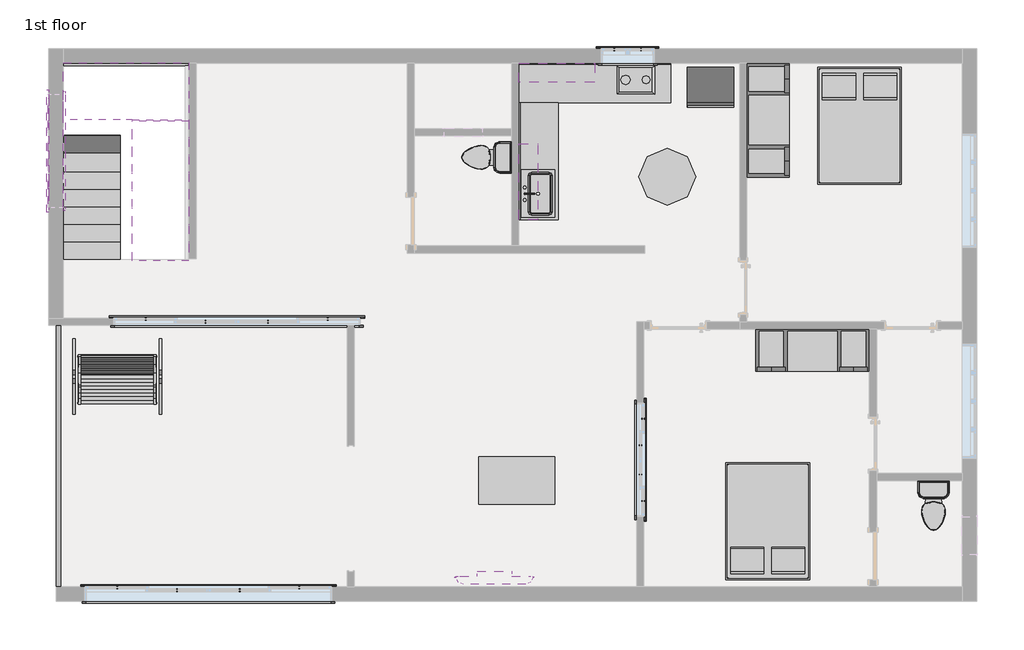
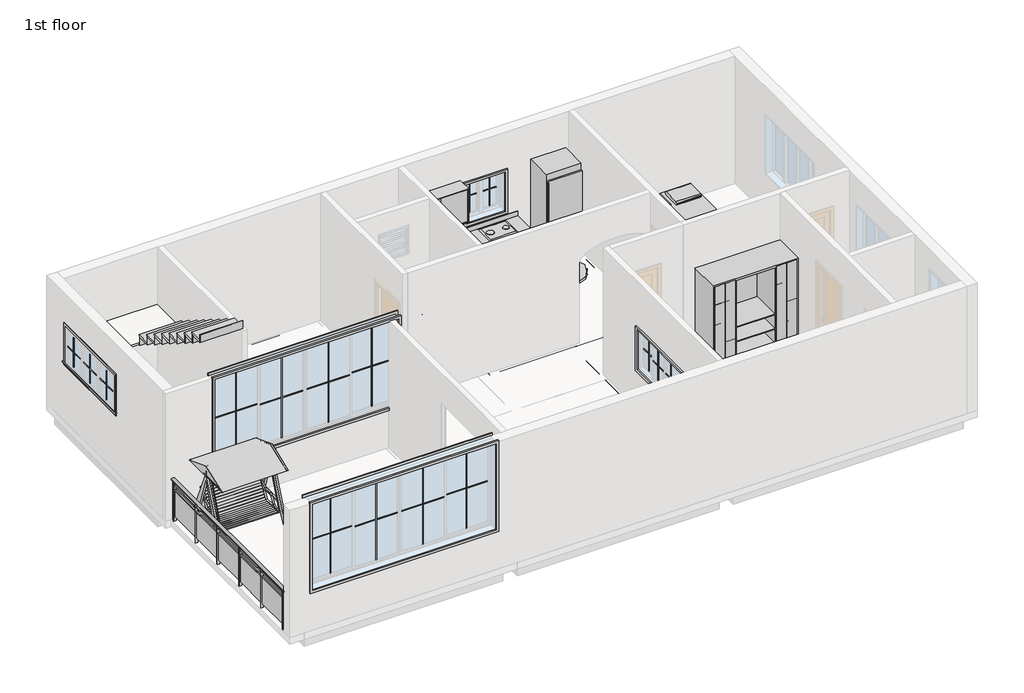
# One storey, part 2 of 2: 30 proxies, 16 furniture elements, 8 beams, 3 flow terminals, 2 stair flights, 1 railing, 1 slab.
"""IFC4 building model written with IfcOpenShell, lengths in millimetres."""

from ifc_helpers import new_model, si_unit, point, frame, origin, place, context, project, spatial, polyline, ellipse_curve, trimmed, outline, extrude, faceted_brep, transform, mapped, element, save
from ifc_brep_helpers import plane_surface, extruded_surface, advanced_brep
from components import proxy_3c1fa1d0, proxy_caef4acf, muntin_pattern_2x2_muntin_pattern_2x2_31a16349, muntin_pattern_2x2_muntin_pattern_2x2_a56fcb99, muntin_pattern_2x2_muntin_pattern_2x2_c58f38d7, muntin_pattern_2x2_muntin_pattern_2x2_b3fe6957, muntin_pattern_2x2_muntin_pattern_2x2_3e0ecaf2, muntin_pattern_2x2_muntin_pattern_2x2_51cb8927, proxy_19935bb1, trim_window_exterior_flat_with_sill_3c945769, trim_window_exterior_flat_with_sill_7b949e88, trim_window_exterior_flat_with_sill_41619996, trim_window_exterior_flat_with_sill_170b7f0e, trim_window_interior_flat_picture_frame_0edfbaa2, trim_window_interior_flat_picture_frame_687edbe0, trim_window_interior_flat_picture_frame_51c85655, trim_window_interior_flat_picture_frame_cc79b2fe, flow_terminal_4d548711, toilet_domestic_3d_toilet_domestic_3d_ba6479b0, toilet_domestic_3d_toilet_domestic_3d_30431060, furniture_0762_x_0762mm_a8fad5e2, furniture_f87f75a4, furniture_97fe820d, furniture_b58f7881, furniture_deb1c5d1, furniture_078eb3f3, furniture_88072bd9, furniture_0b81fedb, furniture_acc2807d, furniture_52f35bf4, furniture_f491f192, non_monolithic_landing_e0ece5e3, stair_flight_342035e6, stair_flight_9be7654d

model = new_model("IFC4")

# Units and contexts
model_context = context("Model", 3, world=origin())
ifc_project = project(units=[si_unit("LENGTHUNIT", "METRE", prefix="MILLI")], contexts=[model_context])

# Site, building, storey
site = spatial("IfcSite", under=ifc_project)
building = spatial("IfcBuilding", under=site)
storey = spatial("IfcBuildingStorey", under=building, Name="1st floor", Elevation=3810.0)

# Beams
placement = place(None, origin())
element("IfcBeam", 1, ObjectType="Concrete-Rectangular Beam", at=placement, inside=storey, context=model_context, shape_type="Brep", body=[
    faceted_brep([(-12643.368339, 9510.993496, 3810.0), (-12643.368339, 9282.393496, 3810.0), (-10681.218339, 9282.393496, 3810.0), (-10452.618339, 9282.393496, 3810.0), (-7176.018339, 9282.393496, 3810.0), (-6947.418339, 9282.393496, 3810.0), (-5499.618339, 9282.393496, 3810.0), (-5271.018339, 9282.393496, 3810.0), (-3492.916739, 9282.393496, 3810.0), (-3264.316739, 9282.393496, 3810.0), (-1842.018339, 9282.393496, 3810.0), (-1613.418339, 9282.393496, 3810.0), (1790.181661, 9282.393496, 3810.0), (1790.181661, 9510.993496, 3810.0), (-1575.318339, 9510.993496, 3810.0), (-1575.318339, 9320.493496, 3810.0), (-1880.118339, 9320.493496, 3810.0), (-1880.118339, 9510.993496, 3810.0), (-6909.318339, 9510.993496, 3810.0), (-6909.318339, 9320.493496, 3810.0), (-7214.118339, 9320.493496, 3810.0), (-7214.118339, 9510.993496, 3810.0), (-10414.518339, 9510.993496, 3810.0), (-10414.518339, 9320.493496, 3810.0), (-10719.318339, 9320.493496, 3810.0), (-10719.318339, 9510.993496, 3810.0), (-12643.368339, 9282.393496, 3505.2), (-10681.218339, 9282.393496, 3505.2), (-10452.618339, 9282.393496, 3505.2), (-7176.018339, 9282.393496, 3505.2), (-6947.418339, 9282.393496, 3505.2), (-5499.618339, 9282.393496, 3505.2), (-5271.018339, 9282.393496, 3505.2), (-3492.916739, 9282.393496, 3505.2), (-3264.316739, 9282.393496, 3505.2), (-1842.018339, 9282.393496, 3505.2), (-1613.418339, 9282.393496, 3505.2), (1790.181661, 9282.393496, 3505.2), (-12643.368339, 9510.993496, 3505.2), (-10719.318339, 9510.993496, 3505.2), (-10719.318339, 9320.493496, 3505.2), (-10414.518339, 9320.493496, 3505.2), (-10414.518339, 9510.993496, 3505.2), (-7214.118339, 9510.993496, 3505.2), (-7214.118339, 9320.493496, 3505.2), (-6909.318339, 9320.493496, 3505.2), (-6909.318339, 9510.993496, 3505.2), (-1880.118339, 9510.993496, 3505.2), (-1880.118339, 9320.493496, 3505.2), (-1575.318339, 9320.493496, 3505.2), (-1575.318339, 9510.993496, 3505.2), (1790.181661, 9510.993496, 3505.2)], [[[0, 1, 2, 3, 4, 5, 6, 7, 8, 9, 10, 11, 12, 13, 14, 15, 16, 17, 18, 19, 20, 21, 22, 23, 24, 25]], [[1, 26, 27, 28, 29, 30, 31, 32, 33, 34, 35, 36, 37, 12, 11, 10, 9, 8, 7, 6, 5, 4, 3, 2]], [[26, 38, 39, 40, 41, 42, 43, 44, 45, 46, 47, 48, 49, 50, 51, 37, 36, 35, 34, 33, 32, 31, 30, 29, 28, 27]], [[13, 51, 50, 14]], [[1, 0, 38, 26]], [[13, 12, 37, 51]], [[41, 23, 22, 42]], [[23, 41, 40, 24]], [[24, 40, 39, 25]], [[38, 0, 25, 39]], [[45, 19, 18, 46]], [[19, 45, 44, 20]], [[20, 44, 43, 21]], [[42, 22, 21, 43]], [[49, 15, 14, 50]], [[15, 49, 48, 16]], [[16, 48, 47, 17]], [[46, 18, 17, 47]]]),
])
element("IfcBeam", 2, ObjectType="Concrete-Rectangular Beam", at=placement, inside=storey, context=model_context, shape_type="Brep", body=[
    faceted_brep([(1790.181661, 913.093496, 3810.0), (2018.781661, 913.093496, 3810.0), (2018.781661, 4958.043496, 3810.0), (1790.181661, 4958.043496, 3810.0), (1790.181661, 2792.693496, 3810.0), (1790.181661, 2564.093496, 3810.0), (1790.181661, 913.093496, 3505.2), (1790.181661, 4958.043496, 3505.2), (1790.181661, 2792.693496, 3505.2), (1790.181661, 2564.093496, 3505.2), (2018.781661, 913.093496, 3505.2), (2018.781661, 4958.043496, 3505.2)], [[[0, 1, 2, 3, 4, 5]], [[6, 0, 5, 4, 3, 7, 8, 9]], [[10, 6, 9, 8, 7, 11]], [[1, 10, 11, 2]], [[1, 0, 6, 10]], [[3, 2, 11, 7]]]),
    faceted_brep([(1790.181661, 9244.293496, 3810.0), (2018.781661, 9244.293496, 3810.0), (2018.781661, 9244.293496, 3505.2), (1790.181661, 9244.293496, 3505.2), (2018.781661, 5262.843496, 3810.0), (1790.181661, 5262.843496, 3810.0), (1790.181661, 5262.843496, 3505.2), (2018.781661, 5262.843496, 3505.2), (1790.181661, 6443.943496, 3810.0), (1790.181661, 6215.343496, 3810.0), (1790.181661, 6443.943496, 3505.2), (1790.181661, 6215.343496, 3505.2)], [[[0, 1, 2, 3]], [[4, 5, 6, 7]], [[1, 0, 8, 9, 5, 4]], [[0, 3, 10, 11, 6, 5, 9, 8]], [[3, 2, 7, 6, 11, 10]], [[2, 1, 4, 7]]]),
])
element("IfcBeam", 3, ObjectType="Concrete-Rectangular Beam", at=placement, inside=storey, context=model_context, shape_type="SweptSolid", body=[
    extrude(outline(polyline([(-6947.418339, 8094.943496), (-6947.418339, 8323.543496), (-5499.618339, 8323.543496), (-5499.618339, 8094.943496), (-6947.418339, 8094.943496)])), frame((0.0, 0.0, 3505.2), z_axis=(0.0, 0.0, 1.0), x_axis=(1.0, 0.0, 0.0)), (0.0, 0.0, 1.0), 304.8),
])
element("IfcBeam", 4, ObjectType="Concrete-Rectangular Beam", at=placement, inside=storey, context=model_context, shape_type="Brep", body=[
    faceted_brep([(-6947.418339, 6443.943496, 3810.0), (-6947.418339, 6215.343496, 3810.0), (-5499.618339, 6215.343496, 3810.0), (-5499.618339, 6443.943496, 3810.0), (-6947.418339, 6215.343496, 3505.2), (-5499.618339, 6215.343496, 3505.2), (-6947.418339, 6443.943496, 3505.2), (-5499.618339, 6443.943496, 3505.2)], [[[0, 1, 2, 3]], [[1, 4, 5, 2]], [[4, 6, 7, 5]], [[6, 0, 3, 7]], [[1, 0, 6, 4]], [[3, 2, 5, 7]]]),
    faceted_brep([(1790.181661, 6443.943496, 3810.0), (1790.181661, 6215.343496, 3810.0), (1790.181661, 6215.343496, 3505.2), (1790.181661, 6443.943496, 3505.2), (-5271.018339, 6215.343496, 3810.0), (-5271.018339, 6443.943496, 3810.0), (-5271.018339, 6443.943496, 3505.2), (-5271.018339, 6215.343496, 3505.2), (-1613.418339, 6443.943496, 3810.0), (-1842.018339, 6443.943496, 3810.0), (-3264.316739, 6443.943496, 3810.0), (-3492.916739, 6443.943496, 3810.0), (-3492.916739, 6215.343496, 3810.0), (-3264.316739, 6215.343496, 3810.0), (-1842.018339, 6215.343496, 3810.0), (-1613.418339, 6215.343496, 3810.0), (-3492.916739, 6215.343496, 3505.2), (-3264.316739, 6215.343496, 3505.2), (-1842.018339, 6215.343496, 3505.2), (-1613.418339, 6215.343496, 3505.2), (-3492.916739, 6443.943496, 3505.2), (-3264.316739, 6443.943496, 3505.2), (-1842.018339, 6443.943496, 3505.2), (-1613.418339, 6443.943496, 3505.2)], [[[0, 1, 2, 3]], [[4, 5, 6, 7]], [[1, 0, 8, 9, 10, 11, 5, 4, 12, 13, 14, 15]], [[2, 1, 15, 14, 13, 12, 4, 7, 16, 17, 18, 19]], [[3, 2, 19, 18, 17, 16, 7, 6, 20, 21, 22, 23]], [[0, 3, 23, 22, 21, 20, 6, 5, 11, 10, 9, 8]]]),
])
element("IfcBeam", 5, ObjectType="Concrete-Rectangular Beam", at=placement, inside=storey, context=model_context, shape_type="Brep", body=[
    faceted_brep([(-1842.018339, 913.093496, 3810.0), (-1613.418339, 913.093496, 3810.0), (-1613.418339, 4996.143496, 3810.0), (-1613.418339, 5224.743496, 3810.0), (-1613.418339, 6215.343496, 3810.0), (-1842.018339, 6215.343496, 3810.0), (-1842.018339, 5281.893496, 3810.0), (-1784.868339, 5281.893496, 3810.0), (-1784.868339, 5053.293496, 3810.0), (-1842.018339, 5053.293496, 3810.0), (-1842.018339, 4996.143496, 3810.0), (-1842.018339, 913.093496, 3505.2), (-1842.018339, 5053.293496, 3505.2), (-1842.018339, 4996.143496, 3505.2), (-1613.418339, 913.093496, 3505.2), (-1784.868339, 5053.293496, 3505.2), (-1784.868339, 5281.893496, 3505.2), (-1842.018339, 5281.893496, 3505.2), (-1842.018339, 6215.343496, 3505.2), (-1613.418339, 6215.343496, 3505.2), (-1613.418339, 5224.743496, 3505.2), (-1613.418339, 4996.143496, 3505.2)], [[[0, 1, 2, 3, 4, 5, 6, 7, 8, 9, 10]], [[11, 0, 10, 9, 12, 13]], [[14, 11, 13, 12, 15, 16, 17, 18, 19, 20, 21]], [[1, 14, 21, 20, 19, 4, 3, 2]], [[1, 0, 11, 14]], [[5, 4, 19, 18]], [[8, 15, 12, 9]], [[16, 7, 6, 17]], [[7, 16, 15, 8]], [[5, 18, 17, 6]]]),
    faceted_brep([(-1842.018339, 9282.393496, 3810.0), (-1613.418339, 9282.393496, 3810.0), (-1613.418339, 9282.393496, 3505.2), (-1842.018339, 9282.393496, 3505.2), (-1613.418339, 6443.943496, 3810.0), (-1842.018339, 6443.943496, 3810.0), (-1842.018339, 6443.943496, 3505.2), (-1613.418339, 6443.943496, 3505.2)], [[[0, 1, 2, 3]], [[4, 5, 6, 7]], [[1, 0, 5, 4]], [[3, 2, 7, 6]], [[2, 1, 4, 7]], [[0, 3, 6, 5]]]),
])
element("IfcBeam", 6, ObjectType="Concrete-Rectangular Beam", at=placement, inside=storey, context=model_context, shape_type="SweptSolid", body=[
    extrude(outline(polyline([(-3492.916739, 9282.393496), (-3264.316739, 9282.393496), (-3264.316739, 6443.943496), (-3492.916739, 6443.943496), (-3492.916739, 9282.393496)])), frame((0.0, 0.0, 3505.2), z_axis=(0.0, 0.0, 1.0), x_axis=(1.0, 0.0, 0.0)), (0.0, 0.0, 1.0), 304.8),
    extrude(outline(polyline([(-3492.916739, 6215.343496), (-3264.316739, 6215.343496), (-3264.316739, 5224.743496), (-3492.916739, 5224.743496), (-3492.916739, 6215.343496)])), frame((0.0, 0.0, 3505.2), z_axis=(0.0, 0.0, 1.0), x_axis=(1.0, 0.0, 0.0)), (0.0, 0.0, 1.0), 304.8),
    extrude(outline(polyline([(-3492.916739, 4996.143496), (-3264.316739, 4996.143496), (-3264.316739, 913.093496), (-3492.916739, 913.093496), (-3492.916739, 4996.143496)])), frame((0.0, 0.0, 3505.2), z_axis=(0.0, 0.0, 1.0), x_axis=(1.0, 0.0, 0.0)), (0.0, 0.0, 1.0), 304.8),
])
element("IfcBeam", 7, ObjectType="Concrete-Rectangular Beam", at=placement, inside=storey, context=model_context, shape_type="Brep", body=[
    faceted_brep([(240.781661, 913.093496, 3810.0), (469.381661, 913.093496, 3810.0), (469.381661, 2564.093496, 3810.0), (469.381661, 2792.693496, 3810.0), (469.381661, 4996.143496, 3810.0), (240.781661, 4996.143496, 3810.0), (469.381661, 913.093496, 3505.2), (469.381661, 2564.093496, 3505.2), (469.381661, 2792.693496, 3505.2), (469.381661, 4996.143496, 3505.2), (240.781661, 913.093496, 3505.2), (240.781661, 4996.143496, 3505.2)], [[[0, 1, 2, 3, 4, 5]], [[1, 6, 7, 8, 9, 4, 3, 2]], [[6, 10, 11, 9, 8, 7]], [[10, 0, 5, 11]], [[1, 0, 10, 6]], [[5, 4, 9, 11]]]),
])
element("IfcBeam", 8, ObjectType="Concrete-Rectangular Beam", at=placement, inside=storey, context=model_context, shape_type="SweptSolid", body=[
    extrude(outline(polyline([(1790.181661, 2792.693496), (1790.181661, 2564.093496), (469.381661, 2564.093496), (469.381661, 2792.693496), (1790.181661, 2792.693496)])), frame((0.0, 0.0, 3505.2), z_axis=(0.0, 0.0, 1.0), x_axis=(1.0, 0.0, 0.0)), (0.0, 0.0, 1.0), 304.8),
])

# Proxies
proxy_shape = proxy_3c1fa1d0(model_context)
element("IfcBuildingElementProxy", 9, Name="Cook Top-2 Unit : 12\" x 18\"", ObjectType="Cook Top-2 Unit : 12\" x 18\"", at=placement, inside=storey, context=model_context, shape_type="MappedRepresentation", body=[
    mapped(proxy_shape, transform((-3421.5185434, 8977.593496, 3810.0), x_axis=(0.0, 1.0, 0.0), y_axis=(-1.0, 0.0, 0.0), z_axis=(0.0, 0.0, 1.0))),
])
proxy_2_shape = proxy_caef4acf(model_context)
element("IfcBuildingElementProxy", 10, Name="Cook Top-2 Unit : 16\" x 22\"", ObjectType="Cook Top-2 Unit : 16\" x 22\"", at=placement, inside=storey, context=model_context, shape_type="MappedRepresentation", body=[
    mapped(proxy_2_shape, transform((-3370.7185434, 8977.593496, 3810.0), x_axis=(0.0, 1.0, 0.0), y_axis=(-1.0, 0.0, 0.0), z_axis=(0.0, 0.0, 1.0))),
])
muntin_pattern_2x2_muntin_pattern_2x2_shape = muntin_pattern_2x2_muntin_pattern_2x2_31a16349(model_context)
element("IfcBuildingElementProxy", 11, Name="Muntin Pattern_2x2 : Muntin Pattern_2x2", ObjectType="Muntin Pattern_2x2 : Muntin Pattern_2x2", at=placement, inside=storey, context=model_context, shape_type="MappedRepresentation", body=[
    mapped(muntin_pattern_2x2_muntin_pattern_2x2_shape, transform((-3330.991739, 3615.018496, 4806.95), x_axis=(0.0, -1.0, 0.0), y_axis=(1.0, 0.0, 0.0), z_axis=(0.0, 0.0, 1.0))),
])
element("IfcBuildingElementProxy", 12, Name="Muntin Pattern_2x2 : Muntin Pattern_2x2", ObjectType="Muntin Pattern_2x2 : Muntin Pattern_2x2", at=placement, inside=storey, context=model_context, shape_type="MappedRepresentation", body=[
    mapped(muntin_pattern_2x2_muntin_pattern_2x2_shape, transform((-3375.441739, 3189.568496, 4806.95), x_axis=(0.0, -1.0, 0.0), y_axis=(1.0, 0.0, 0.0), z_axis=(0.0, 0.0, 1.0))),
])
element("IfcBuildingElementProxy", 13, Name="Muntin Pattern_2x2 : Muntin Pattern_2x2", ObjectType="Muntin Pattern_2x2 : Muntin Pattern_2x2", at=placement, inside=storey, context=model_context, shape_type="MappedRepresentation", body=[
    mapped(muntin_pattern_2x2_muntin_pattern_2x2_shape, transform((-3375.441739, 2719.668496, 4806.95), x_axis=(0.0, -1.0, 0.0), y_axis=(1.0, 0.0, 0.0), z_axis=(0.0, 0.0, 1.0))),
])
element("IfcBuildingElementProxy", 14, Name="Muntin Pattern_2x2 : Muntin Pattern_2x2", ObjectType="Muntin Pattern_2x2 : Muntin Pattern_2x2", at=placement, inside=storey, context=model_context, shape_type="MappedRepresentation", body=[
    mapped(muntin_pattern_2x2_muntin_pattern_2x2_shape, transform((-3330.991739, 2294.218496, 4806.95), x_axis=(0.0, -1.0, 0.0), y_axis=(1.0, 0.0, 0.0), z_axis=(0.0, 0.0, 1.0))),
])
muntin_pattern_2x2_muntin_pattern_2x2_2_shape = muntin_pattern_2x2_muntin_pattern_2x2_a56fcb99(model_context)
element("IfcBuildingElementProxy", 15, Name="Muntin Pattern_2x2 : Muntin Pattern_2x2", ObjectType="Muntin Pattern_2x2 : Muntin Pattern_2x2", at=placement, inside=storey, context=model_context, shape_type="MappedRepresentation", body=[
    mapped(muntin_pattern_2x2_muntin_pattern_2x2_2_shape, transform((-12862.443339, 7303.3101627, 5251.45), x_axis=(0.0, 1.0, 0.0), y_axis=(-1.0, 0.0, 0.0), z_axis=(0.0, 0.0, 1.0))),
])
element("IfcBuildingElementProxy", 16, Name="Muntin Pattern_2x2 : Muntin Pattern_2x2", ObjectType="Muntin Pattern_2x2 : Muntin Pattern_2x2", at=placement, inside=storey, context=model_context, shape_type="MappedRepresentation", body=[
    mapped(muntin_pattern_2x2_muntin_pattern_2x2_2_shape, transform((-12862.443339, 7910.793496, 5251.45), x_axis=(0.0, 1.0, 0.0), y_axis=(-1.0, 0.0, 0.0), z_axis=(0.0, 0.0, 1.0))),
])
muntin_pattern_2x2_muntin_pattern_2x2_3_shape = muntin_pattern_2x2_muntin_pattern_2x2_c58f38d7(model_context)
element("IfcBuildingElementProxy", 17, Name="Muntin Pattern_2x2 : Muntin Pattern_2x2", ObjectType="Muntin Pattern_2x2 : Muntin Pattern_2x2", at=placement, inside=storey, context=model_context, shape_type="MappedRepresentation", body=[
    mapped(muntin_pattern_2x2_muntin_pattern_2x2_3_shape, transform((-12862.443339, 8518.2768293, 5251.45), x_axis=(0.0, -1.0, 0.0), y_axis=(1.0, 0.0, 0.0), z_axis=(0.0, 0.0, 1.0))),
])
muntin_pattern_2x2_muntin_pattern_2x2_4_shape = muntin_pattern_2x2_muntin_pattern_2x2_b3fe6957(model_context)
element("IfcBuildingElementProxy", 18, Name="Muntin Pattern_2x2 : Muntin Pattern_2x2", ObjectType="Muntin Pattern_2x2 : Muntin Pattern_2x2", at=placement, inside=storey, context=model_context, shape_type="MappedRepresentation", body=[
    mapped(muntin_pattern_2x2_muntin_pattern_2x2_4_shape, transform((-3796.230839, 9539.568496, 4984.75), x_axis=(1.0, 0.0, 0.0), y_axis=(0.0, 1.0, 0.0), z_axis=(0.0, 0.0, 1.0))),
])
muntin_pattern_2x2_muntin_pattern_2x2_5_shape = muntin_pattern_2x2_muntin_pattern_2x2_3e0ecaf2(model_context)
element("IfcBuildingElementProxy", 19, Name="Muntin Pattern_2x2 : Muntin Pattern_2x2", ObjectType="Muntin Pattern_2x2 : Muntin Pattern_2x2", at=placement, inside=storey, context=model_context, shape_type="MappedRepresentation", body=[
    mapped(muntin_pattern_2x2_muntin_pattern_2x2_5_shape, transform((-3367.605839, 9539.568496, 4984.75), x_axis=(-1.0, 0.0, 0.0), y_axis=(0.0, -1.0, 0.0), z_axis=(0.0, 0.0, 1.0))),
])
muntin_pattern_2x2_muntin_pattern_2x2_6_shape = muntin_pattern_2x2_muntin_pattern_2x2_51cb8927(model_context)
element("IfcBuildingElementProxy", 20, Name="Muntin Pattern_2x2 : Muntin Pattern_2x2", ObjectType="Muntin Pattern_2x2 : Muntin Pattern_2x2", at=placement, inside=storey, context=model_context, shape_type="MappedRepresentation", body=[
    mapped(muntin_pattern_2x2_muntin_pattern_2x2_6_shape, transform((-11316.218339, 5215.218496, 4806.95), x_axis=(1.0, 0.0, 0.0), y_axis=(0.0, 1.0, 0.0), z_axis=(0.0, 0.0, 1.0))),
])
element("IfcBuildingElementProxy", 21, Name="Muntin Pattern_2x2 : Muntin Pattern_2x2", ObjectType="Muntin Pattern_2x2 : Muntin Pattern_2x2", at=placement, inside=storey, context=model_context, shape_type="MappedRepresentation", body=[
    mapped(muntin_pattern_2x2_muntin_pattern_2x2_6_shape, transform((-10357.368339, 5170.768496, 4806.95), x_axis=(1.0, 0.0, 0.0), y_axis=(0.0, 1.0, 0.0), z_axis=(0.0, 0.0, 1.0))),
])
element("IfcBuildingElementProxy", 22, Name="Muntin Pattern_2x2 : Muntin Pattern_2x2", ObjectType="Muntin Pattern_2x2 : Muntin Pattern_2x2", at=placement, inside=storey, context=model_context, shape_type="MappedRepresentation", body=[
    mapped(muntin_pattern_2x2_muntin_pattern_2x2_6_shape, transform((-9354.068339, 5170.768496, 4806.95), x_axis=(1.0, 0.0, 0.0), y_axis=(0.0, 1.0, 0.0), z_axis=(0.0, 0.0, 1.0))),
])
element("IfcBuildingElementProxy", 23, Name="Muntin Pattern_2x2 : Muntin Pattern_2x2", ObjectType="Muntin Pattern_2x2 : Muntin Pattern_2x2", at=placement, inside=storey, context=model_context, shape_type="MappedRepresentation", body=[
    mapped(muntin_pattern_2x2_muntin_pattern_2x2_6_shape, transform((-8395.218339, 5215.218496, 4806.95), x_axis=(1.0, 0.0, 0.0), y_axis=(0.0, 1.0, 0.0), z_axis=(0.0, 0.0, 1.0))),
])
element("IfcBuildingElementProxy", 24, Name="Muntin Pattern_2x2 : Muntin Pattern_2x2", ObjectType="Muntin Pattern_2x2 : Muntin Pattern_2x2", at=placement, inside=storey, context=model_context, shape_type="MappedRepresentation", body=[
    mapped(muntin_pattern_2x2_muntin_pattern_2x2_6_shape, transform((-11773.418339, 903.568496, 4806.95), x_axis=(1.0, 0.0, 0.0), y_axis=(0.0, 1.0, 0.0), z_axis=(0.0, 0.0, 1.0))),
])
element("IfcBuildingElementProxy", 25, Name="Muntin Pattern_2x2 : Muntin Pattern_2x2", ObjectType="Muntin Pattern_2x2 : Muntin Pattern_2x2", at=placement, inside=storey, context=model_context, shape_type="MappedRepresentation", body=[
    mapped(muntin_pattern_2x2_muntin_pattern_2x2_6_shape, transform((-10814.568339, 859.118496, 4806.95), x_axis=(1.0, 0.0, 0.0), y_axis=(0.0, 1.0, 0.0), z_axis=(0.0, 0.0, 1.0))),
])
element("IfcBuildingElementProxy", 26, Name="Muntin Pattern_2x2 : Muntin Pattern_2x2", ObjectType="Muntin Pattern_2x2 : Muntin Pattern_2x2", at=placement, inside=storey, context=model_context, shape_type="MappedRepresentation", body=[
    mapped(muntin_pattern_2x2_muntin_pattern_2x2_6_shape, transform((-9811.268339, 859.118496, 4806.95), x_axis=(1.0, 0.0, 0.0), y_axis=(0.0, 1.0, 0.0), z_axis=(0.0, 0.0, 1.0))),
])
element("IfcBuildingElementProxy", 27, Name="Muntin Pattern_2x2 : Muntin Pattern_2x2", ObjectType="Muntin Pattern_2x2 : Muntin Pattern_2x2", at=placement, inside=storey, context=model_context, shape_type="MappedRepresentation", body=[
    mapped(muntin_pattern_2x2_muntin_pattern_2x2_6_shape, transform((-8852.418339, 903.568496, 4806.95), x_axis=(1.0, 0.0, 0.0), y_axis=(0.0, 1.0, 0.0), z_axis=(0.0, 0.0, 1.0))),
])
proxy_3_shape = proxy_19935bb1(model_context)
element("IfcBuildingElementProxy", 28, Name="Refrigerator-Built-in : 30\" x 24\" LH", ObjectType="Refrigerator-Built-in : 30\" x 24\" LH", at=placement, inside=storey, context=model_context, shape_type="MappedRepresentation", body=[
    mapped(proxy_3_shape, transform((-2254.768339, 8966.8695245, 3810.0), x_axis=(1.0, 0.0, 0.0), y_axis=(0.0, 1.0, 0.0), z_axis=(0.0, 0.0, 1.0))),
])
trim_window_exterior_flat_with_sill_shape = trim_window_exterior_flat_with_sill_3c945769(model_context)
element("IfcBuildingElementProxy", 29, Name="Trim-Window-Exterior-Flat : with Sill", ObjectType="Trim-Window-Exterior-Flat : with Sill", at=placement, inside=storey, context=model_context, shape_type="MappedRepresentation", body=[
    mapped(trim_window_exterior_flat_with_sill_shape, transform((-3321.466739, 2954.618496, 5638.8), x_axis=(0.0, 1.0, 0.0), y_axis=(0.0, 0.0, 1.0), z_axis=(1.0, 0.0, 0.0))),
])
trim_window_exterior_flat_with_sill_2_shape = trim_window_exterior_flat_with_sill_7b949e88(model_context)
element("IfcBuildingElementProxy", 30, Name="Trim-Window-Exterior-Flat : with Sill", ObjectType="Trim-Window-Exterior-Flat : with Sill", at=placement, inside=storey, context=model_context, shape_type="MappedRepresentation", body=[
    mapped(trim_window_exterior_flat_with_sill_2_shape, transform((-12871.968339, 7910.793496, 5994.4), x_axis=(0.0, 1.0, 0.0), y_axis=(0.0, 0.0, -1.0), z_axis=(-1.0, 0.0, 0.0))),
])
trim_window_exterior_flat_with_sill_3_shape = trim_window_exterior_flat_with_sill_41619996(model_context)
element("IfcBuildingElementProxy", 31, Name="Trim-Window-Exterior-Flat : with Sill", ObjectType="Trim-Window-Exterior-Flat : with Sill", at=placement, inside=storey, context=model_context, shape_type="MappedRepresentation", body=[
    mapped(trim_window_exterior_flat_with_sill_3_shape, transform((-3581.918339, 9549.093496, 5829.3), x_axis=(-1.0, 0.0, 0.0), y_axis=(0.0, 0.0, 1.0), z_axis=(0.0, 1.0, 0.0))),
])
trim_window_exterior_flat_with_sill_4_shape = trim_window_exterior_flat_with_sill_170b7f0e(model_context)
element("IfcBuildingElementProxy", 32, Name="Trim-Window-Exterior-Flat : with Sill", ObjectType="Trim-Window-Exterior-Flat : with Sill", at=placement, inside=storey, context=model_context, shape_type="MappedRepresentation", body=[
    mapped(trim_window_exterior_flat_with_sill_4_shape, transform((-9855.718339, 5224.743496, 6705.6), x_axis=(-1.0, 0.0, 0.0), y_axis=(0.0, 0.0, 1.0), z_axis=(0.0, 1.0, 0.0))),
])
element("IfcBuildingElementProxy", 33, Name="Trim-Window-Exterior-Flat : with Sill", ObjectType="Trim-Window-Exterior-Flat : with Sill", at=placement, inside=storey, context=model_context, shape_type="MappedRepresentation", body=[
    mapped(trim_window_exterior_flat_with_sill_4_shape, transform((-10312.918339, 913.093496, 6705.6), x_axis=(-1.0, 0.0, 0.0), y_axis=(0.0, 0.0, 1.0), z_axis=(0.0, 1.0, 0.0))),
])
trim_window_interior_flat_picture_frame_shape = trim_window_interior_flat_picture_frame_0edfbaa2(model_context)
element("IfcBuildingElementProxy", 34, Name="Trim-Window-Interior-Flat : Picture Frame", ObjectType="Trim-Window-Interior-Flat : Picture Frame", at=placement, inside=storey, context=model_context, shape_type="MappedRepresentation", body=[
    mapped(trim_window_interior_flat_picture_frame_shape, transform((-3435.766739, 2954.618496, 5638.8), x_axis=(0.0, -1.0, 0.0), y_axis=(0.0, 0.0, 1.0), z_axis=(-1.0, 0.0, 0.0))),
])
trim_window_interior_flat_picture_frame_2_shape = trim_window_interior_flat_picture_frame_687edbe0(model_context)
element("IfcBuildingElementProxy", 35, Name="Trim-Window-Interior-Flat : Picture Frame", ObjectType="Trim-Window-Interior-Flat : Picture Frame", at=placement, inside=storey, context=model_context, shape_type="MappedRepresentation", body=[
    mapped(trim_window_interior_flat_picture_frame_2_shape, transform((-12643.368339, 7910.793496, 5994.4), x_axis=(0.0, -1.0, 0.0), y_axis=(0.0, 0.0, -1.0), z_axis=(1.0, 0.0, 0.0))),
])
trim_window_interior_flat_picture_frame_3_shape = trim_window_interior_flat_picture_frame_51c85655(model_context)
element("IfcBuildingElementProxy", 36, Name="Trim-Window-Interior-Flat : Picture Frame", ObjectType="Trim-Window-Interior-Flat : Picture Frame", at=placement, inside=storey, context=model_context, shape_type="MappedRepresentation", body=[
    mapped(trim_window_interior_flat_picture_frame_3_shape, transform((-3581.918339, 9320.493496, 5829.3), x_axis=(1.0, 0.0, 0.0), y_axis=(0.0, 0.0, 1.0), z_axis=(0.0, -1.0, 0.0))),
])
trim_window_interior_flat_picture_frame_4_shape = trim_window_interior_flat_picture_frame_cc79b2fe(model_context)
element("IfcBuildingElementProxy", 37, Name="Trim-Window-Interior-Flat : Picture Frame", ObjectType="Trim-Window-Interior-Flat : Picture Frame", at=placement, inside=storey, context=model_context, shape_type="MappedRepresentation", body=[
    mapped(trim_window_interior_flat_picture_frame_4_shape, transform((-9855.718339, 5110.443496, 6705.6), x_axis=(1.0, 0.0, 0.0), y_axis=(0.0, 0.0, 1.0), z_axis=(0.0, -1.0, 0.0))),
])
element("IfcBuildingElementProxy", 38, Name="Trim-Window-Interior-Flat : Picture Frame", ObjectType="Trim-Window-Interior-Flat : Picture Frame", at=placement, inside=storey, context=model_context, shape_type="MappedRepresentation", body=[
    mapped(trim_window_interior_flat_picture_frame_4_shape, transform((-10312.918339, 684.493496, 6705.6), x_axis=(1.0, 0.0, 0.0), y_axis=(0.0, 0.0, 1.0), z_axis=(0.0, -1.0, 0.0))),
])

# Flow terminals
flow_terminal_shape = flow_terminal_4d548711(model_context)
element("IfcFlowTerminal", 39, ObjectType="Sink Kitchen-Single : 30\" x 21\"", at=placement, inside=storey, context=model_context, shape_type="MappedRepresentation", body=[
    mapped(flow_terminal_shape, transform((-5021.0229378, 7209.3042554, 3810.0), x_axis=(0.0, 1.0, 0.0), y_axis=(-1.0, 0.0, 0.0), z_axis=(0.0, 0.0, 1.0))),
])
toilet_domestic_3d_toilet_domestic_3d_shape = toilet_domestic_3d_toilet_domestic_3d_ba6479b0(model_context)
toilet_domestic_3d_toilet_domestic_3d_2_shape = toilet_domestic_3d_toilet_domestic_3d_30431060(model_context)
element("IfcFlowTerminal", 40, ObjectType="Toilet-Domestic-3D : Toilet-Domestic-3D", at=placement, inside=storey, context=model_context, shape_type="MappedRepresentation", body=[
    mapped(toilet_domestic_3d_toilet_domestic_3d_shape, transform((-5937.1643663, 7809.6710196, 3810.0), x_axis=(0.0, -1.0, 0.0), y_axis=(1.0, 0.0, 0.0), z_axis=(0.0, 0.0, 1.0))),
    mapped(toilet_domestic_3d_toilet_domestic_3d_2_shape, transform((-5937.1643663, 7809.6710196, 3810.0), x_axis=(0.0, -1.0, 0.0), y_axis=(1.0, 0.0, 0.0), z_axis=(0.0, 0.0, 1.0))),
])
element("IfcFlowTerminal", 41, ObjectType="Toilet-Domestic-3D : Toilet-Domestic-3D", at=placement, inside=storey, context=model_context, shape_type="MappedRepresentation", body=[
    mapped(toilet_domestic_3d_toilet_domestic_3d_shape, transform((1325.531896, 2126.5474686, 3810.0), x_axis=(1.0, 0.0, 0.0), y_axis=(0.0, 1.0, 0.0), z_axis=(0.0, 0.0, 1.0))),
    mapped(toilet_domestic_3d_toilet_domestic_3d_2_shape, transform((1325.531896, 2126.5474686, 3810.0), x_axis=(1.0, 0.0, 0.0), y_axis=(0.0, 1.0, 0.0), z_axis=(0.0, 0.0, 1.0))),
])

# Furniture
furniture_0762_x_0762mm_shape = furniture_0762_x_0762mm_a8fad5e2(model_context)
element("IfcFurniture", 42, ObjectType="0762 x 0762mm", at=placement, inside=storey, context=model_context, shape_type="MappedRepresentation", body=[
    mapped(furniture_0762_x_0762mm_shape, transform((-12213.2088951, 3373.8694389, 3810.0), x_axis=(1.0, 0.0, 0.0), y_axis=(0.0, 1.0, 0.0), z_axis=(0.0, 0.0, 1.0))),
])
furniture_shape = furniture_f87f75a4(model_context)
element("IfcFurniture", 43, ObjectType="Base Cabinet-Combo01 : 30\"", at=placement, inside=storey, context=model_context, shape_type="MappedRepresentation", body=[
    mapped(furniture_shape, transform((-4051.5060439, 9320.493496, 3810.0), x_axis=(1.0, 0.0, 0.0), y_axis=(0.0, 1.0, 0.0), z_axis=(0.0, 0.0, 1.0))),
])
element("IfcFurniture", 44, ObjectType="Base Cabinet-Combo01 : 30\"", at=placement, inside=storey, context=model_context, shape_type="MappedRepresentation", body=[
    mapped(furniture_shape, transform((-5328.168339, 8006.3557911, 3810.0), x_axis=(0.0, 1.0, 0.0), y_axis=(-1.0, 0.0, 0.0), z_axis=(0.0, 0.0, 1.0))),
])
element("IfcFurniture", 45, ObjectType="Base Cabinet-Combo01 : 30\"", at=placement, inside=storey, context=model_context, shape_type="MappedRepresentation", body=[
    mapped(furniture_shape, transform((-3289.5060439, 9320.493496, 3810.0), x_axis=(1.0, 0.0, 0.0), y_axis=(0.0, 1.0, 0.0), z_axis=(0.0, 0.0, 1.0))),
])
furniture_2_shape = furniture_97fe820d(model_context)
element("IfcFurniture", 46, ObjectType="Base Cabinet-Corner Unit-Square : 36\"", at=placement, inside=storey, context=model_context, shape_type="MappedRepresentation", body=[
    mapped(furniture_2_shape, transform((-5328.168339, 8793.7557911, 3810.0), x_axis=(0.0, 1.0, 0.0), y_axis=(-1.0, 0.0, 0.0), z_axis=(0.0, 0.0, 1.0))),
])
furniture_3_shape = furniture_b58f7881(model_context)
element("IfcFurniture", 47, ObjectType="Bed-Box : Double 53\" x 74\"", at=placement, inside=storey, context=model_context, shape_type="MappedRepresentation", body=[
    mapped(furniture_3_shape, transform((-199.970798, 8551.6230042, 3810.0), x_axis=(1.0, 0.0, 0.0), y_axis=(0.0, 1.0, 0.0), z_axis=(0.0, 0.0, 1.0))),
])
element("IfcFurniture", 48, ObjectType="Bed-Box : Double 53\" x 74\"", at=placement, inside=storey, context=model_context, shape_type="MappedRepresentation", body=[
    mapped(furniture_3_shape, transform((-994.7642799, 1732.7639878, 3810.0), x_axis=(-1.0, 0.0, 0.0), y_axis=(0.0, -1.0, 0.0), z_axis=(0.0, 0.0, 1.0))),
])
furniture_4_shape = furniture_deb1c5d1(model_context)
element("IfcFurniture", 49, ObjectType="Counter Top : 24\" Depth", at=placement, inside=storey, context=model_context, shape_type="MappedRepresentation", body=[
    mapped(furniture_4_shape, transform((-4127.7060439, 9320.493496, 3810.0), x_axis=(1.0, 0.0, 0.0), y_axis=(0.0, 1.0, 0.0), z_axis=(0.0, 0.0, 1.0))),
])
furniture_5_shape = furniture_078eb3f3(model_context)
element("IfcFurniture", 50, ObjectType="Counter Top w Sink Hole : 24\" Depth", at=placement, inside=storey, context=model_context, shape_type="MappedRepresentation", body=[
    mapped(furniture_5_shape, transform((-5328.168339, 8006.6364215, 3810.0), x_axis=(0.0, 1.0, 0.0), y_axis=(-1.0, 0.0, 0.0), z_axis=(0.0, 0.0, 1.0))),
])
furniture_6_shape = furniture_88072bd9(model_context)
element("IfcFurniture", 51, ObjectType="Entertainment Center.0001 : 72\" x 72\" x 24\"", at=placement, inside=storey, context=model_context, shape_type="MappedRepresentation", body=[
    mapped(furniture_6_shape, transform((-616.468339, 5154.893496, 3810.0), x_axis=(1.0, 0.0, 0.0), y_axis=(0.0, 1.0, 0.0), z_axis=(0.0, 0.0, 1.0))),
])
element("IfcFurniture", 52, ObjectType="Entertainment Center.0001 : 72\" x 72\" x 24\"", at=placement, inside=storey, context=model_context, shape_type="MappedRepresentation", body=[
    mapped(furniture_6_shape, transform((-1772.168339, 8406.093496, 3810.0), x_axis=(0.0, 1.0, 0.0), y_axis=(-1.0, 0.0, 0.0), z_axis=(0.0, 0.0, 1.0))),
])
furniture_7_shape = furniture_0b81fedb(model_context)
element("IfcFurniture", 53, ObjectType="TV - Flat Screen : 50\"", at=placement, inside=storey, context=model_context, shape_type="MappedRepresentation", body=[
    mapped(furniture_7_shape, transform((-5725.8128531, 1013.6142575, 5029.2), x_axis=(-1.0, 0.0, 0.0), y_axis=(0.0, -1.0, 0.0), z_axis=(0.0, 0.0, 1.0))),
])
furniture_8_shape = furniture_acc2807d(model_context)
element("IfcFurniture", 54, ObjectType="Table-Coffee Rectangular : 48\" x 30\"", at=placement, inside=storey, context=model_context, shape_type="MappedRepresentation", body=[
    mapped(furniture_8_shape, transform((-5973.1503692, 2251.6326642, 3810.0), x_axis=(1.0, 0.0, 0.0), y_axis=(0.0, 1.0, 0.0), z_axis=(0.0, 0.0, 1.0))),
])
furniture_9_shape = furniture_52f35bf4(model_context)
element("IfcFurniture", 55, ObjectType="Table-Dining Round w Chairs : 36\" Diameter", at=placement, inside=storey, context=model_context, shape_type="MappedRepresentation", body=[
    mapped(furniture_9_shape, transform((-3050.6003062, 7682.9221845, 3810.0), x_axis=(1.0, 0.0, 0.0), y_axis=(0.0, 1.0, 0.0), z_axis=(0.0, 0.0, 1.0))),
])
furniture_10_shape = furniture_f491f192(model_context)
element("IfcFurniture", 56, ObjectType="Upper Cabinet-Pass-Thru w Glass : 48\" x 30\" x 12\"", at=placement, inside=storey, context=model_context, shape_type="MappedRepresentation", body=[
    mapped(furniture_10_shape, transform((-4737.3060439, 9320.493496, 3810.0), x_axis=(1.0, 0.0, 0.0), y_axis=(0.0, 1.0, 0.0), z_axis=(0.0, 0.0, 1.0))),
])
element("IfcFurniture", 57, ObjectType="Upper Cabinet-Pass-Thru w Glass : 48\" x 30\" x 12\"", at=placement, inside=storey, context=model_context, shape_type="MappedRepresentation", body=[
    mapped(furniture_10_shape, transform((-5328.168339, 7397.0364215, 3810.0), x_axis=(0.0, 1.0, 0.0), y_axis=(-1.0, 0.0, 0.0), z_axis=(0.0, 0.0, 1.0))),
])

# Railing
element("IfcRailing", 58, ObjectType="Glass Panel - Bottom Fill", at=placement, inside=storey, context=model_context, shape_type="SolidModel", body=[
    advanced_brep(
    [(-12681.468339, 5110.443496, 4724.4), (-12757.668339, 5110.443496, 4724.4), (-12681.468339, 913.093496, 4724.4), (-12757.668339, 913.093496, 4724.4)],
    [
        (0, 1, ellipse_curve(frame((-12719.568339, 5110.443496, 4724.4), z_axis=(0.0, 1.0, 0.0), x_axis=(-1.0, 0.0, 0.0)), 38.1, 28.575)),
        (1, 0, ellipse_curve(frame((-12719.568339, 5110.443496, 4724.4), z_axis=(0.0, 1.0, 0.0), x_axis=(-1.0, 0.0, 0.0)), 38.1, 28.575)),
        (2, 3, ellipse_curve(frame((-12719.568339, 913.093496, 4724.4), z_axis=(0.0, -1.0, 0.0), x_axis=(-1.0, 0.0, 0.0)), 38.1, 28.575)),
        (3, 2, ellipse_curve(frame((-12719.568339, 913.093496, 4724.4), z_axis=(0.0, -1.0, 0.0), x_axis=(-1.0, 0.0, 0.0)), 38.1, 28.575)),
        (0, 2),
        (3, 1),
    ],
    [
        plane_surface(frame((-12719.568339, 5110.443496, 4724.4), z_axis=(0.0, 1.0, 0.0), x_axis=(0.0, 0.0, -1.0))),
        plane_surface(frame((-12719.568339, 913.093496, 4724.4), z_axis=(0.0, -1.0, 0.0), x_axis=(0.0, 0.0, -1.0))),
        extruded_surface(trimmed(ellipse_curve(frame((-12719.568339, 913.093496, 4724.4), z_axis=(0.0, 1.0, 0.0), x_axis=(-1.0, 0.0, 0.0)), 38.1, 28.575), [point((-12681.468339, 913.093496, 4724.4))], [point((-12757.668339, 913.093496, 4724.4))], True, "CARTESIAN"), (0.0, 4197.35, 0.0), 4197.35),
        extruded_surface(trimmed(ellipse_curve(frame((-12719.568339, 913.093496, 4724.4), z_axis=(0.0, 1.0, 0.0), x_axis=(-1.0, 0.0, 0.0)), 38.1, 28.575), [point((-12757.668339, 913.093496, 4724.4))], [point((-12681.468339, 913.093496, 4724.4))], True, "CARTESIAN"), (0.0, 4197.35, 0.0), 4197.35),
    ],
    [
        (0, [[1, 2]]),
        (1, [[3, 4]]),
        (2, [[-1, 5, -4, 6]]),
        (3, [[-2, -6, -3, -5]]),
    ],
),
    extrude(outline(polyline([(-12732.268339, 5110.443496), (-12706.868339, 5110.443496), (-12706.868339, 913.093496), (-12732.268339, 913.093496), (-12732.268339, 5110.443496)])), frame((0.0, 0.0, 4610.1), z_axis=(0.0, 0.0, 1.0), x_axis=(1.0, 0.0, 0.0)), (0.0, 0.0, 1.0), 25.4),
    extrude(outline(polyline([(-12732.268339, 5110.443496), (-12706.868339, 5110.443496), (-12706.868339, 913.093496), (-12732.268339, 913.093496), (-12732.268339, 5110.443496)])), frame((0.0, 0.0, 4508.5), z_axis=(0.0, 0.0, 1.0), x_axis=(1.0, 0.0, 0.0)), (0.0, 0.0, 1.0), 25.4),
    extrude(outline(polyline([(-12744.968339, 986.118496), (-12694.168339, 986.118496), (-12694.168339, 973.418496), (-12744.968339, 973.418496), (-12744.968339, 986.118496)])), frame((0.0, 0.0, 3810.0), z_axis=(0.0, 0.0, 1.0), x_axis=(1.0, 0.0, 0.0)), (0.0, 0.0, 1.0), 885.825),
    extrude(outline(polyline([(-12713.0331819, 1792.568496), (-12713.0331819, 979.768496), (-12719.3831819, 979.768496), (-12719.3831819, 1792.568496), (-12713.0331819, 1792.568496)])), frame((0.0, 0.0, 3911.6), z_axis=(0.0, 0.0, 1.0), x_axis=(1.0, 0.0, 0.0)), (0.0, 0.0, 1.0), 596.9),
    extrude(outline(polyline([(-12744.968339, 1798.918496), (-12694.168339, 1798.918496), (-12694.168339, 1786.218496), (-12744.968339, 1786.218496), (-12744.968339, 1798.918496)])), frame((0.0, 0.0, 3810.0), z_axis=(0.0, 0.0, 1.0), x_axis=(1.0, 0.0, 0.0)), (0.0, 0.0, 1.0), 885.825),
    extrude(outline(polyline([(-12713.0331819, 2605.368496), (-12713.0331819, 1792.568496), (-12719.3831819, 1792.568496), (-12719.3831819, 2605.368496), (-12713.0331819, 2605.368496)])), frame((0.0, 0.0, 3911.6), z_axis=(0.0, 0.0, 1.0), x_axis=(1.0, 0.0, 0.0)), (0.0, 0.0, 1.0), 596.9),
    extrude(outline(polyline([(-12744.968339, 2611.718496), (-12694.168339, 2611.718496), (-12694.168339, 2599.018496), (-12744.968339, 2599.018496), (-12744.968339, 2611.718496)])), frame((0.0, 0.0, 3810.0), z_axis=(0.0, 0.0, 1.0), x_axis=(1.0, 0.0, 0.0)), (0.0, 0.0, 1.0), 885.825),
    extrude(outline(polyline([(-12713.0331819, 3418.168496), (-12713.0331819, 2605.368496), (-12719.3831819, 2605.368496), (-12719.3831819, 3418.168496), (-12713.0331819, 3418.168496)])), frame((0.0, 0.0, 3911.6), z_axis=(0.0, 0.0, 1.0), x_axis=(1.0, 0.0, 0.0)), (0.0, 0.0, 1.0), 596.9),
    extrude(outline(polyline([(-12744.968339, 3424.518496), (-12694.168339, 3424.518496), (-12694.168339, 3411.818496), (-12744.968339, 3411.818496), (-12744.968339, 3424.518496)])), frame((0.0, 0.0, 3810.0), z_axis=(0.0, 0.0, 1.0), x_axis=(1.0, 0.0, 0.0)), (0.0, 0.0, 1.0), 885.825),
    extrude(outline(polyline([(-12713.0331819, 4230.968496), (-12713.0331819, 3418.168496), (-12719.3831819, 3418.168496), (-12719.3831819, 4230.968496), (-12713.0331819, 4230.968496)])), frame((0.0, 0.0, 3911.6), z_axis=(0.0, 0.0, 1.0), x_axis=(1.0, 0.0, 0.0)), (0.0, 0.0, 1.0), 596.9),
    extrude(outline(polyline([(-12744.968339, 4237.318496), (-12694.168339, 4237.318496), (-12694.168339, 4224.618496), (-12744.968339, 4224.618496), (-12744.968339, 4237.318496)])), frame((0.0, 0.0, 3810.0), z_axis=(0.0, 0.0, 1.0), x_axis=(1.0, 0.0, 0.0)), (0.0, 0.0, 1.0), 885.825),
    extrude(outline(polyline([(-12713.0331819, 5043.768496), (-12713.0331819, 4230.968496), (-12719.3831819, 4230.968496), (-12719.3831819, 5043.768496), (-12713.0331819, 5043.768496)])), frame((0.0, 0.0, 3911.6), z_axis=(0.0, 0.0, 1.0), x_axis=(1.0, 0.0, 0.0)), (0.0, 0.0, 1.0), 596.9),
    extrude(outline(polyline([(-12744.968339, 5050.118496), (-12694.168339, 5050.118496), (-12694.168339, 5037.418496), (-12744.968339, 5037.418496), (-12744.968339, 5050.118496)])), frame((0.0, 0.0, 3810.0), z_axis=(0.0, 0.0, 1.0), x_axis=(1.0, 0.0, 0.0)), (0.0, 0.0, 1.0), 885.825),
    extrude(outline(polyline([(-12729.093339, 925.793496), (-12710.043339, 925.793496), (-12710.043339, 906.743496), (-12729.093339, 906.743496), (-12729.093339, 925.793496)])), frame((0.0, 0.0, 3810.0), z_axis=(0.0, 0.0, 1.0), x_axis=(1.0, 0.0, 0.0)), (0.0, 0.0, 1.0), 885.825),
    extrude(outline(polyline([(-12729.093339, 5116.793496), (-12710.043339, 5116.793496), (-12710.043339, 5097.743496), (-12729.093339, 5097.743496), (-12729.093339, 5116.793496)])), frame((0.0, 0.0, 3810.0), z_axis=(0.0, 0.0, 1.0), x_axis=(1.0, 0.0, 0.0)), (0.0, 0.0, 1.0), 885.825),
])

# Slab
non_monolithic_landing_shape = non_monolithic_landing_e0ece5e3(model_context)
element("IfcSlab", 59, ObjectType="Non-Monolithic Landing", at=placement, inside=storey, context=model_context, shape_type="MappedRepresentation", body=[
    mapped(non_monolithic_landing_shape, transform((0.0, 0.0, 0.0), x_axis=(1.0, 0.0, 0.0), y_axis=(0.0, 1.0, 0.0), z_axis=(0.0, 0.0, 1.0))),
])

# Stair flights
stair_flight_shape = stair_flight_342035e6(model_context)
element("IfcStairFlight", 60, ObjectType="2\" Tread 1\" Nosing 1/4\" Riser", at=placement, inside=storey, context=model_context, shape_type="MappedRepresentation", body=[
    mapped(stair_flight_shape, transform((0.0, 0.0, 0.0), x_axis=(1.0, 0.0, 0.0), y_axis=(0.0, 1.0, 0.0), z_axis=(0.0, 0.0, 1.0))),
])
stair_flight_2_shape = stair_flight_9be7654d(model_context)
element("IfcStairFlight", 61, ObjectType="2\" Tread 1\" Nosing 1/4\" Riser", at=placement, inside=storey, context=model_context, shape_type="MappedRepresentation", body=[
    mapped(stair_flight_2_shape, transform((0.0, 0.0, 0.0), x_axis=(1.0, 0.0, 0.0), y_axis=(0.0, 1.0, 0.0), z_axis=(0.0, 0.0, 1.0))),
])

save(model, "model.ifc")

# Revit data of these elements
# Type "Concrete-Rectangular Beam"
#   Assembly Code = "B10"
#   Length [instance default] = 5 ft
#   b = 0.75 ft
#   h = 1 ft
#   Structural Material [instance default] = Concrete, Cast-in-Place gray
# Type "Cook Top-2 Unit : 12\" x 18\""
#   Assembly Code = "E1090400"
#   Counter Height = 3 ft
#   Depth = 2 ft
#   Width = 1.5 ft
#   Burner Material = Metal - Chrome
#   Cooktop Material = Metal - Steel, Polished
#   Default Elevation = 0
# Type "Cook Top-2 Unit : 16\" x 22\""
#   Assembly Code = "E1090400"
#   Counter Height = 2.583333 ft
#   Depth = 1.833333 ft
#   Width = 1.333333 ft
#   Burner Material = Metal - Chrome
#   Cooktop Material = Metal - Steel, Polished
#   Default Elevation = 0
# Type "Muntin Pattern_2x2 : Muntin Pattern_2x2"
#   Width [instance default] = 4 ft
#   Thickness = 0.041667 ft
#   Height [instance default] = 4 ft
#   Distance = 0.0625 ft
#   Interior Material [instance default] = none
#   Exterior Material [instance default] = none
#   Default Elevation = 0
# Type "Refrigerator-Built-in : 30\" x 24\" LH"
#   Assembly Code = "E1090400"
#   Depth = 2 ft
#   Handle = 0.020833 ft
#   Height = 7 ft
#   Top Door Height = 5 ft
#   Width = 2.458333 ft
#   Material = Metal - Paint Finish - Ivory,Glossy
#   Default Elevation = 0
# Type "Trim-Window-Exterior-Flat : with Sill"
#   Trim Width = 0.1875 ft
#   Trim Thickness_Picture Frame = 0.104167 ft
#   Trim Thickness_with Sill = 0.0625 ft
#   Sill Thickness = 0.104167 ft
#   Opening Width [instance default] = 2 ft
#   Opening Height [instance default] = 3 ft
#   Default Elevation = 4 ft
#   Sill = yes
#   Picture Frame = no
#   Trim Material [instance default] = none
# Type "Trim-Window-Interior-Flat : Picture Frame"
#   Trim Thickness_Picture Frame = 0.104167 ft
#   Trim Width = 0.1875 ft
#   Trim Thickness_with Sill = 0.0625 ft
#   Sill Thickness = 0.104167 ft
#   Opening Width [instance default] = 2 ft
#   Opening Height [instance default] = 3 ft
#   Default Elevation = 4 ft
#   Sill = no
#   Picture Frame = yes
#   Trim Material [instance default] = none
# Type "Sink Kitchen-Single : 30\" x 21\""
#   Assembly Code = "D2010410"
#   Counter Height = 3 ft
#   Depth = 1.75 ft
#   Width = 2.5 ft
#   Faucet Material = Steel, Polished
#   Sink Material = Steel, Polished
#   Default Elevation = 0
# Type "Toilet-Domestic-3D : Toilet-Domestic-3D"
#   Assembly Code = "D2010110"
#   Toilet - Bowl/Basin Material = Porcelain, Linen
#   Toilet - Seat Material = Laminate, Linen, Matte
#   Default Elevation = 0
# Type "0762 x 0762mm"
#   Height = 1.499344 ft
#   Length = 2.5 ft
#   Width = 2.5 ft
#   Base Material = Wood - Birch
#   Top Material = Laminate - Ivory, Matte
#   Default Elevation = 0
# Type "Base Cabinet-Combo01 : 30\""
#   Depth = 1.833333 ft
#   Height = 2.979167 ft
#   Toe Depth = 0.25 ft
#   Toe Height = 0.291667 ft
#   Width = 2.5 ft
#   Default Elevation = 0
# Type "Base Cabinet-Corner Unit-Square : 36\""
#   Assembly Code = "C1030410"
#   Depth = 2 ft
#   Height = 2.875 ft
#   Toe Depth = 0.25 ft
#   Toe Height = 0.291667 ft
#   Width = 3 ft
#   Cabinet Material = Cabinets
#   Door/Drawer Material = Cabinets
#   Handle Material = Cabinets - Handles
#   Default Elevation = 0
# Type "Bed-Box : Double 53\" x 74\""
#   Assembly Code = "E2020200"
#   Length = 6.166667 ft
#   Width = 4.416667 ft
#   Frame Material = Birch
#   Mattress Material = Linen, White
#   Default Elevation = 0
# Type "Counter Top : 24\" Depth"
#   Assembly Code = "C1030400"
#   Counter Thickness = 0.125 ft
#   Depth = 2.083333 ft
#   Height = 3 ft
#   Length [instance default] = 8 ft
#   Counter Top Material = none
#   Default Elevation = 0
# Type "Counter Top w Sink Hole : 24\" Depth"
#   Assembly Code = "C1030400"
#   Counter Thickness = 0.125 ft
#   Depth = 2.083333 ft
#   Height = 3 ft
#   Length [instance default] = 8 ft
#   Sink Location [instance default] = 2 ft
#   Sink Location To Wall [instance default] = 0.5 ft
#   Sink Opening Depth [instance default] = 1.25 ft
#   Sink Opening Width [instance default] = 2.25 ft
#   Counter Top Material = none
#   Default Elevation = 0
# Type "Entertainment Center.0001 : 72\" x 72\" x 24\""
#   Assembly Code = "E2020200"
#   Center Width = 2.666667 ft
#   Depth = 2 ft
#   Height = 6 ft
#   Width = 6 ft
#   Material = none
#   Default Elevation = 0
# Type "TV - Flat Screen : 50\""
#   SinAng = 0.001609 ft
#   L = 3.631485 ft
#   H = 2.042898 ft
#   Thickness = 0.360892 ft
#   Diagonal = 4.166667 ft
#   CosAng = 0.002859 ft
#   Stand [instance default] = yes
#   Default Elevation = 0
# Type "Table-Coffee Rectangular : 48\" x 30\""
#   Assembly Code = "E2020200"
#   Height = 1.083333 ft
#   Length = 4 ft
#   Width = 2.5 ft
#   Base Material = Metal - Chrome
#   Table Top Material = Glass - Clear, Grey
#   Default Elevation = 0
# Type "Table-Dining Round w Chairs : 36\" Diameter"
#   Assembly Code = "E2020200"
#   Radius = 1.5 ft
#   Diameter = 3 ft
#   Height = 2.5 ft
#   Chairs = 6
#   Base Material = Pine
#   Top Material = Laminate, Linen, Matte
#   Default Elevation = 0
# Type "Upper Cabinet-Pass-Thru w Glass : 48\" x 30\" x 12\""
#   Depth = 1 ft
#   Height = 2.5 ft
#   Top Of Cabinet = 7 ft
#   Width = 4 ft
#   Default Elevation = 0
# Type "Glass Panel - Bottom Fill"
#   Assembly Code = "C2010400"
#   built-in parameter 1008612 = 0.0416667 (stored number, unit not read)
#   built-in parameter 1008611 = 0.0416667 (stored number, unit not read)
#   built-in parameter 1008609 = 0.333333 (stored number, unit not read)
#   built-in parameter 1008604 = 0.166667 (stored number, unit not read)
#   built-in parameter 1008603 = 0.166667 (stored number, unit not read)
#   Railing Height = 3 ft
#   built-in parameter 1008630 = 2
#   built-in parameter 1008610 = 2
#   built-in parameter 1008618 = Baluster - Square : 3/4"
# Elements 1, 2, 3, 4, 5, 6, 7, 8 (IfcBeam, "Concrete-Rectangular Beam")
#   Structural Material = Concrete, Cast-in-Place gray
#   Phase Created = New Construction
#   Materials on its faces: "Concrete, Cast-in-Place gray"
# Element 9 (IfcBuildingElementProxy, "Cook Top-2 Unit : 12\" x 18\"")
#   Phase Created = New Construction
#   Materials on its faces: "Metal - Steel, Polished", "Metal - Chrome"
# Element 10 (IfcBuildingElementProxy, "Cook Top-2 Unit : 16\" x 22\"")
#   Phase Created = New Construction
#   Materials on its faces: "Metal - Steel, Polished", "Metal - Chrome"
# Elements 11, 12, 13, 14 (IfcBuildingElementProxy, "Muntin Pattern_2x2 : Muntin Pattern_2x2")
#   Width = 1.25 ft
#   Height = 2.520833 ft
#   Interior Material = Wood - Stained
#   Exterior Material = Clad - White
#   Phase Created = New Construction
#   Materials on its faces: "Clad - White", "Wood - Stained"
# Elements 15, 16, 17 (IfcBuildingElementProxy, "Muntin Pattern_2x2 : Muntin Pattern_2x2")
#   Width = 1.555556 ft
#   Height = 2.208333 ft
#   Interior Material = Wood - Stained
#   Exterior Material = Clad - White
#   Phase Created = New Construction
#   Materials on its faces: "Clad - White", "Wood - Stained"
# Elements 18, 19 (IfcBuildingElementProxy, "Muntin Pattern_2x2 : Muntin Pattern_2x2")
#   Width = 0.96875 ft
#   Height = 2.541667 ft
#   Interior Material = Wood - Stained
#   Exterior Material = Clad - White
#   Phase Created = New Construction
#   Materials on its faces: "Clad - White", "Wood - Stained"
# Elements 20, 21, 22, 23, 24, 25, 26, 27 (IfcBuildingElementProxy, "Muntin Pattern_2x2 : Muntin Pattern_2x2")
#   Width = 3 ft
#   Height = 6.020833 ft
#   Interior Material = Wood - Stained
#   Exterior Material = Clad - White
#   Phase Created = New Construction
#   Materials on its faces: "Clad - White", "Wood - Stained"
# Element 28 (IfcBuildingElementProxy, "Refrigerator-Built-in : 30\" x 24\" LH")
#   Phase Created = New Construction
#   Materials on its faces: "Metal - Paint Finish - Ivory,Glossy", "Metal - Chrome"
# Element 29 (IfcBuildingElementProxy, "Trim-Window-Exterior-Flat : with Sill")
#   Opening Width = 6 ft
#   Opening Height = 3 ft
#   Trim Material = Clad - White
#   Phase Created = New Construction
#   Materials on its faces: "Clad - White"
# Element 30 (IfcBuildingElementProxy, "Trim-Window-Exterior-Flat : with Sill")
#   Opening Width = 6 ft
#   Opening Height = 2.666667 ft
#   Trim Material = Clad - White
#   Phase Created = New Construction
#   Materials on its faces: "Clad - White"
# Element 31 (IfcBuildingElementProxy, "Trim-Window-Exterior-Flat : with Sill")
#   Opening Width = 2.833333 ft
#   Opening Height = 3 ft
#   Trim Material = Clad - White
#   Phase Created = New Construction
#   Materials on its faces: "Clad - White"
# Elements 32, 33 (IfcBuildingElementProxy, "Trim-Window-Exterior-Flat : with Sill")
#   Opening Width = 13 ft
#   Opening Height = 6.5 ft
#   Trim Material = Clad - White
#   Phase Created = New Construction
#   Materials on its faces: "Clad - White"
# Element 34 (IfcBuildingElementProxy, "Trim-Window-Interior-Flat : Picture Frame")
#   Opening Width = 6 ft
#   Opening Height = 3 ft
#   Trim Material = Wood - Stained
#   Phase Created = New Construction
#   Materials on its faces: "Wood - Stained"
# Element 35 (IfcBuildingElementProxy, "Trim-Window-Interior-Flat : Picture Frame")
#   Opening Width = 6 ft
#   Opening Height = 2.666667 ft
#   Trim Material = Wood - Stained
#   Phase Created = New Construction
#   Materials on its faces: "Wood - Stained"
# Element 36 (IfcBuildingElementProxy, "Trim-Window-Interior-Flat : Picture Frame")
#   Opening Width = 2.833333 ft
#   Opening Height = 3 ft
#   Trim Material = Wood - Stained
#   Phase Created = New Construction
#   Materials on its faces: "Wood - Stained"
# Elements 37, 38 (IfcBuildingElementProxy, "Trim-Window-Interior-Flat : Picture Frame")
#   Opening Width = 13 ft
#   Opening Height = 6.5 ft
#   Trim Material = Wood - Stained
#   Phase Created = New Construction
#   Materials on its faces: "Wood - Stained"
# Element 39 (IfcFlowTerminal, "Sink Kitchen-Single : 30\" x 21\"")
#   Mark = "4"
#   Phase Created = New Construction
#   Materials on its faces: "Steel, Polished"
# Element 40 (IfcFlowTerminal, "Toilet-Domestic-3D : Toilet-Domestic-3D")
#   Mark = "5"
#   Phase Created = New Construction
#   Materials on its faces: "Porcelain, Linen", "Laminate, Linen, Matte"
# Element 41 (IfcFlowTerminal, "Toilet-Domestic-3D : Toilet-Domestic-3D")
#   Mark = "6"
#   Phase Created = New Construction
#   Materials on its faces: "Porcelain, Linen", "Laminate, Linen, Matte"
# Element 42 (IfcFurniture, "0762 x 0762mm")
#   Phase Created = New Construction
#   Materials on its faces: "wood finish", "steel", "Laminate - Ivory, Matte", "fabric"
# Elements 43, 44, 45 (IfcFurniture, "Base Cabinet-Combo01 : 30\"")
#   Phase Created = New Construction
#   Materials on its faces: "Cabinet"
# Element 46 (IfcFurniture, "Base Cabinet-Corner Unit-Square : 36\"")
#   Phase Created = New Construction
#   Materials on its faces: "Cabinets", "Cabinets - Handles"
# Elements 47, 48 (IfcFurniture, "Bed-Box : Double 53\" x 74\"")
#   Phase Created = New Construction
#   Materials on its faces: "Birch", "Linen, White"
# Element 49 (IfcFurniture, "Counter Top : 24\" Depth")
#   Length = 8 ft
#   Phase Created = New Construction
#   Materials on its faces: "Counter Top"
# Element 50 (IfcFurniture, "Counter Top w Sink Hole : 24\" Depth")
#   Sink Opening Width = 2.25 ft
#   Sink Opening Depth = 1.25 ft
#   Sink Location To Wall = 0.5 ft
#   Sink Location = 1.374079 ft
#   Length = 6.165746 ft
#   Phase Created = New Construction
#   Materials on its faces: "Counter Top"
# Elements 51, 52 (IfcFurniture, "Entertainment Center.0001 : 72\" x 72\" x 24\"")
#   Phase Created = New Construction
#   Materials on its faces: "Steel, Chrome Plated", "Glass - Clear, Grey"
# Element 53 (IfcFurniture, "TV - Flat Screen : 50\"")
#   Stand = yes
#   Phase Created = New Construction
#   Materials on its faces: "TV - Black", "TV - Glass", "TV - Screen"
# Element 54 (IfcFurniture, "Table-Coffee Rectangular : 48\" x 30\"")
#   Phase Created = New Construction
#   Materials on its faces: "Metal - Chrome", "Glass - Clear, Grey"
# Element 55 (IfcFurniture, "Table-Dining Round w Chairs : 36\" Diameter")
#   Phase Created = New Construction
#   Materials on its faces: "Pine", "Laminate, Linen, Matte"
# Elements 56, 57 (IfcFurniture, "Upper Cabinet-Pass-Thru w Glass : 48\" x 30\" x 12\"")
#   Phase Created = New Construction
#   Materials on its faces: "Glass", "Cabinet"
# Element 58 (IfcRailing, "Glass Panel - Bottom Fill")
#   Phase Created = New Construction
#   Materials on its faces: "Glass"
# Element 59 (IfcSlab, "Non-Monolithic Landing")
#   Phase Created = New Construction
# Elements 60, 61 (IfcStairFlight, "2\" Tread 1\" Nosing 1/4\" Riser")
#   Phase Created = New Construction
# Materials
#   "Concrete, Cast-in-Place gray": class "Concrete", colour RGB 192 192 192, transparency 0, Description = "Cast-in-place concrete", Cost = 0
#   "Metal - Chrome": class "Metal", colour RGB 247 247 247, transparency 0
#   "Metal - Steel, Polished": colour RGB 57 57 57, transparency 0
#   "Metal - Paint Finish - Ivory,Glossy": colour RGB 247 247 239, transparency 0
#   "Steel, Polished": class "Metal", colour RGB 57 57 57, transparency 0, Description = "Polished steel", Cost = 0
#   "Porcelain, Linen": class "Ceramic", colour RGB 249 239 230, transparency 0, Description = "Porcelain, linen", Cost = 0
